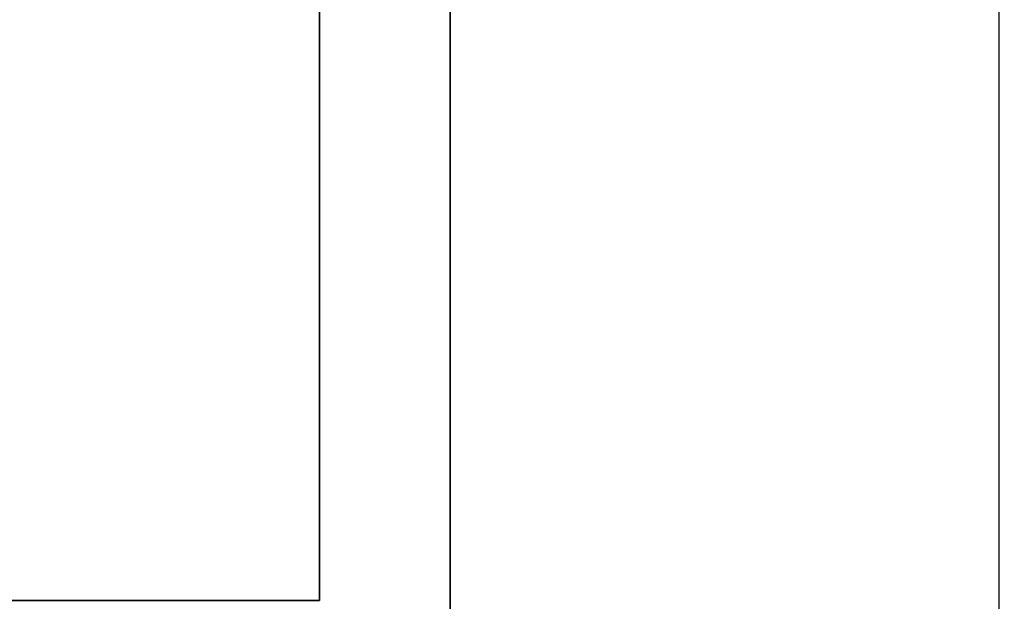
# Model space of a CAD drawing. Units: inches. Extents: x -128 to 854, y -395 to 398.
# Tile 45 of 61: x 284 to 352, y 196 to 236. Entities that reach past the tile are written whole.
import ezdxf

# ---------------------------------------------------------------- set-up
doc = ezdxf.new("R2010")
doc.units = ezdxf.units.IN
doc.header["$MEASUREMENT"] = 0
doc.layers.add('A-ANNO-DIMS', color=2, linetype='Continuous', lineweight=18)
doc.layers.add('A-WALL', color=4, linetype='Continuous', lineweight=35)
doc.styles.get("Standard").update_dxf_attribs({"font": 'arial.ttf'})
doc.dimstyles.get("Standard").update_dxf_attribs({"dimtxt": 0.18, "dimasz": 0.18, "dimexe": 0.18, "dimexo": 0.0625, "dimgap": 0.09, "dimtad": 0, "dimtih": 1, "dimtoh": 1, "dimdec": 1, "dimzin": 0, "dimdsep": 46, "dimlunit": 4, "dimtxsty": 'Standard', "dimcen": 0.09, "dimclrd": 1, "dimclre": 2, "dimclrt": 6, "dimadec": 0, "dimazin": 0, "dimtfac": 1, "dimtdec": 1, "dimtofl": 0, "dimtmove": 0, "dimatfit": 3, "dimfxl": 1, "dimtfill": 2, "dimtfillclr": 3, "dimtolj": 1, "dimtzin": 0, "dimarcsym": 0})

# ---------------------------------------------------------------- blocks, each defined once
blk = doc.blocks.new('*D53')
at = {"layer": 'A-ANNO-DIMS', "color": 0, "lineweight": -2, "transparency": 16777216}
for p, q in [((304.81, 339.741), (280.297, 339.741)), ((280.477, 334.741), (280.477, 269.839)), ((280.477, 200.741), (280.477, 265.642)), ((304.81, 195.741), (280.297, 195.741))]:
    blk.add_line(p, q, dxfattribs=at)
at = {"layer": 'A-ANNO-DIMS', "color": 0, "transparency": 16777216}
for points in [[(279.644, 334.741), (281.311, 334.741), (280.477, 339.741)], [(279.644, 200.741), (281.311, 200.741), (280.477, 195.741)]]:
    blk.add_solid(points, dxfattribs=at)
at = {"layer": 'Defpoints', "color": 0, "transparency": 16777216}
for p in [(280.477, 339.741), (304.873, 339.741), (304.873, 195.741)]:
    blk.add_point(p, dxfattribs=at)
at = {"layer": 'A-ANNO-DIMS', "color": 0, "transparency": 16777216, "insert": (280.477, 267.741), "char_height": 4, "attachment_point": 5, "bg_fill": 1, "box_fill_scale": 1.25, "bg_fill_color": 3, "bg_fill_transparency": 0}
blk.add_mtext("\\A1;12'", dxfattribs=at)
blk = doc.blocks.new('*D98')
at = {"layer": 'A-ANNO-DIMS', "color": 2, "lineweight": -2, "transparency": 16777216}
for p, q in [((313.935, 348.741), (351.853, 348.741)), ((313.935, -89.259), (351.853, -89.259))]:
    blk.add_line(p, q, dxfattribs=at)
at = {"layer": 'A-ANNO-DIMS', "color": 1, "lineweight": -2, "transparency": 16777216}
for p, q in [((351.673, 348.561), (351.673, 129.923)), ((351.673, -89.079), (351.673, 129.559))]:
    blk.add_line(p, q, dxfattribs=at)
at = {"layer": 'A-ANNO-DIMS', "color": 1, "transparency": 16777216}
for points in [[(351.643, 348.561), (351.703, 348.561), (351.673, 348.741)], [(351.643, -89.079), (351.703, -89.079), (351.673, -89.259)]]:
    blk.add_solid(points, dxfattribs=at)
at = {"layer": 'Defpoints', "color": 0, "transparency": 16777216}
for p in [(313.873, 348.741), (351.673, 348.741), (313.873, -89.259)]:
    blk.add_point(p, dxfattribs=at)
at = {"layer": 'A-ANNO-DIMS', "color": 6, "transparency": 16777216, "insert": (351.673, 129.741), "char_height": 0.18, "attachment_point": 5, "bg_fill": 1, "box_fill_scale": 1.25, "bg_fill_color": 3, "bg_fill_transparency": 0}
blk.add_mtext('\\A1;36\'-6"', dxfattribs=at)

msp = doc.modelspace()

# ---------------------------------------------------------------- linework, layer by layer
at = {"layer": 'A-WALL'}
for p, q in [((313.873, 348.741), (313.873, -89.259)), ((304.873, 339.741), (304.873, 195.741)), ((304.873, 195.741), (220.76, 195.741))]:
    msp.add_line(p, q, dxfattribs=at)

# ---------------------------------------------------------------- dimensions: what is measured, and where the dimension line sits
at = {"layer": 'A-ANNO-DIMS'}
for base, p1, p2, override, picture, middle in [((351.673, 348.741), (313.873, -89.259), (313.873, 348.741), {"dimdec": 1, "dimlfac": 1, "dimrnd": 0, "dimzin": 1, "dimdsep": 46, "dimlunit": 4, "dimfrac": 2}, '*D98', (351.673, 129.741)), ((280.477, 339.741), (304.873, 195.741), (304.873, 339.741), {"dimtxt": 4, "dimasz": 5, "dimclrd": 0, "dimclre": 0, "dimclrt": 0}, '*D53', (280.477, 267.741))]:
    dim = msp.add_linear_dim(base=base, p1=p1, p2=p2, angle=90, dimstyle='Standard', override=override, dxfattribs=at)
    dim.commit()
    dim.dimension.update_dxf_attribs({"geometry": picture, "text_midpoint": middle})

doc.saveas('drawing.dxf')
